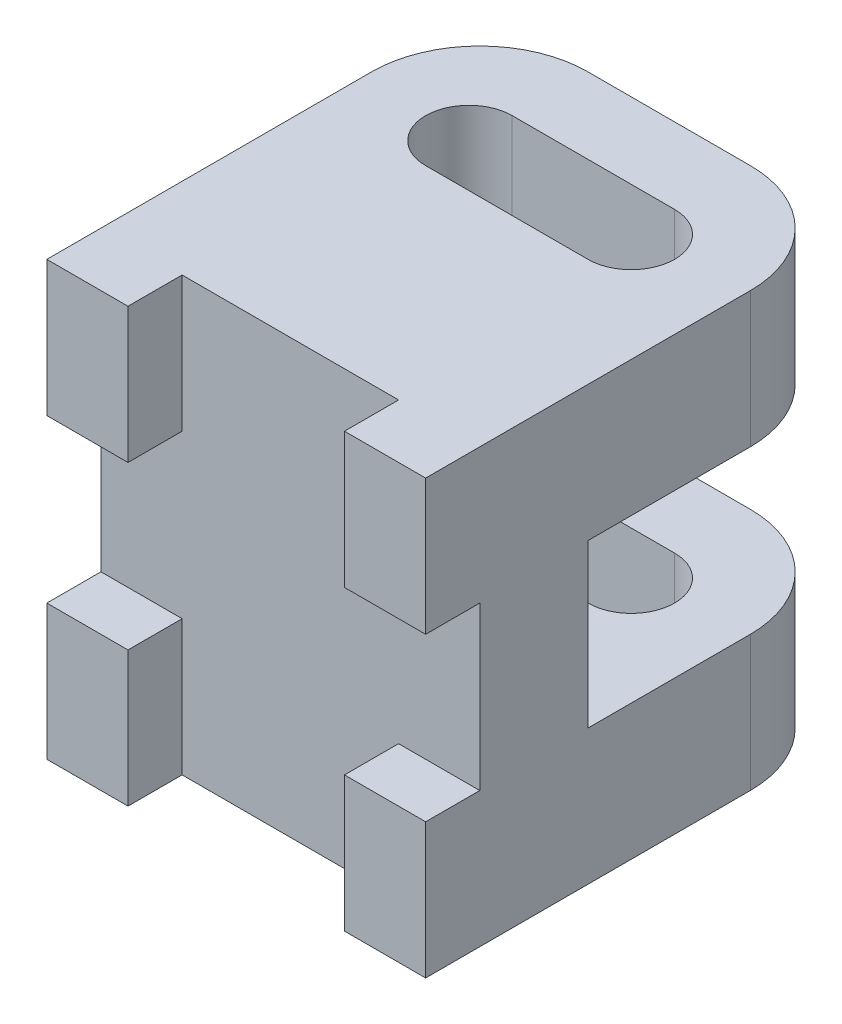
ISO-10303-21;
HEADER;
FILE_DESCRIPTION(('STEP AP214'),'2;1');
FILE_NAME('part.step','',(''),(''),'','','');
FILE_SCHEMA(('AUTOMOTIVE_DESIGN { 1 0 10303 214 1 1 1 1 }'));
ENDSEC;
DATA;
#1=APPLICATION_CONTEXT('core data for automotive mechanical design processes');
#2=APPLICATION_PROTOCOL_DEFINITION('international standard','automotive_design',2000,#1);
#3=PRODUCT_CONTEXT('',#1,'mechanical');
#4=PRODUCT('Part','Part','',(#3));
#5=PRODUCT_RELATED_PRODUCT_CATEGORY('part','',(#4));
#6=PRODUCT_DEFINITION_FORMATION('','',#4);
#7=PRODUCT_DEFINITION_CONTEXT('part definition',#1,'design');
#8=PRODUCT_DEFINITION('design','',#6,#7);
#9=PRODUCT_DEFINITION_SHAPE('','',#8);
#10=(LENGTH_UNIT() NAMED_UNIT(*) SI_UNIT(.MILLI.,.METRE.));
#11=(NAMED_UNIT(*) PLANE_ANGLE_UNIT() SI_UNIT($,.RADIAN.));
#12=(NAMED_UNIT(*) SI_UNIT($,.STERADIAN.) SOLID_ANGLE_UNIT());
#13=UNCERTAINTY_MEASURE_WITH_UNIT(LENGTH_MEASURE(1.E-05),#10,'distance_accuracy_value','');
#14=(GEOMETRIC_REPRESENTATION_CONTEXT(3) GLOBAL_UNCERTAINTY_ASSIGNED_CONTEXT((#13)) GLOBAL_UNIT_ASSIGNED_CONTEXT((#10,
#11,#12)) REPRESENTATION_CONTEXT('',''));
#15=CARTESIAN_POINT('',(0.,0.,0.));
#16=DIRECTION('',(0.,0.,1.));
#17=DIRECTION('',(1.,0.,0.));
#18=AXIS2_PLACEMENT_3D('',#15,#16,#17);
#19=CARTESIAN_POINT('',(0.,80.,20.));
#20=DIRECTION('',(1.,0.,0.));
#21=DIRECTION('',(0.,0.,-1.));
#22=AXIS2_PLACEMENT_3D('',#19,#20,#21);
#23=PLANE('',#22);
#24=DIRECTION('',(0.,-1.,0.));
#25=VECTOR('',#24,1.);
#26=CARTESIAN_POINT('',(0.,100.,-30.));
#27=LINE('',#26,#25);
#28=CARTESIAN_POINT('',(0.,25.,-30.));
#29=VERTEX_POINT('',#28);
#30=CARTESIAN_POINT('',(0.,0.,-30.));
#31=VERTEX_POINT('',#30);
#32=EDGE_CURVE('E506',#29,#31,#27,.T.);
#33=ORIENTED_EDGE('',*,*,#32,.T.);
#34=DIRECTION('',(0.,0.,-1.));
#35=VECTOR('',#34,1.);
#36=CARTESIAN_POINT('',(0.,0.,20.));
#37=LINE('',#36,#35);
#38=CARTESIAN_POINT('',(0.,0.,30.));
#39=VERTEX_POINT('',#38);
#40=EDGE_CURVE('E267',#39,#31,#37,.T.);
#41=ORIENTED_EDGE('',*,*,#40,.F.);
#42=DIRECTION('',(0.,-1.,0.));
#43=VECTOR('',#42,1.);
#44=CARTESIAN_POINT('',(0.,25.,30.));
#45=LINE('',#44,#43);
#46=CARTESIAN_POINT('',(0.,25.,30.));
#47=VERTEX_POINT('',#46);
#48=EDGE_CURVE('E356',#47,#39,#45,.T.);
#49=ORIENTED_EDGE('',*,*,#48,.F.);
#50=DIRECTION('',(0.,0.,-1.));
#51=VECTOR('',#50,1.);
#52=CARTESIAN_POINT('',(0.,25.,30.));
#53=LINE('',#52,#51);
#54=CARTESIAN_POINT('',(0.,25.,20.));
#55=VERTEX_POINT('',#54);
#56=EDGE_CURVE('E369',#47,#55,#53,.T.);
#57=ORIENTED_EDGE('',*,*,#56,.T.);
#58=DIRECTION('',(0.,-1.,0.));
#59=VECTOR('',#58,1.);
#60=CARTESIAN_POINT('',(0.,80.,20.));
#61=LINE('',#60,#59);
#62=CARTESIAN_POINT('',(0.,55.,20.));
#63=VERTEX_POINT('',#62);
#64=EDGE_CURVE('E405',#63,#55,#61,.T.);
#65=ORIENTED_EDGE('',*,*,#64,.F.);
#66=DIRECTION('',(0.,0.,-1.));
#67=VECTOR('',#66,1.);
#68=CARTESIAN_POINT('',(0.,55.,30.));
#69=LINE('',#68,#67);
#70=CARTESIAN_POINT('',(0.,55.,30.));
#71=VERTEX_POINT('',#70);
#72=EDGE_CURVE('E398',#71,#63,#69,.T.);
#73=ORIENTED_EDGE('',*,*,#72,.F.);
#74=DIRECTION('',(0.,-1.,0.));
#75=VECTOR('',#74,1.);
#76=CARTESIAN_POINT('',(0.,80.,30.));
#77=LINE('',#76,#75);
#78=CARTESIAN_POINT('',(0.,80.,30.));
#79=VERTEX_POINT('',#78);
#80=EDGE_CURVE('E380',#79,#71,#77,.T.);
#81=ORIENTED_EDGE('',*,*,#80,.F.);
#82=DIRECTION('',(0.,0.,-1.));
#83=VECTOR('',#82,1.);
#84=CARTESIAN_POINT('',(0.,80.,20.));
#85=LINE('',#84,#83);
#86=CARTESIAN_POINT('',(0.,80.,-30.));
#87=VERTEX_POINT('',#86);
#88=EDGE_CURVE('E414',#79,#87,#85,.T.);
#89=ORIENTED_EDGE('',*,*,#88,.T.);
#90=CARTESIAN_POINT('',(0.,55.,-30.));
#91=VERTEX_POINT('',#90);
#92=EDGE_CURVE('E499',#87,#91,#27,.T.);
#93=ORIENTED_EDGE('',*,*,#92,.T.);
#94=DIRECTION('',(0.,0.,1.));
#95=VECTOR('',#94,1.);
#96=CARTESIAN_POINT('',(0.,55.,-50.));
#97=LINE('',#96,#95);
#98=CARTESIAN_POINT('',(0.,55.,0.));
#99=VERTEX_POINT('',#98);
#100=EDGE_CURVE('E288',#91,#99,#97,.T.);
#101=ORIENTED_EDGE('',*,*,#100,.T.);
#102=DIRECTION('',(0.,-1.,0.));
#103=VECTOR('',#102,1.);
#104=CARTESIAN_POINT('',(0.,80.,0.));
#105=LINE('',#104,#103);
#106=CARTESIAN_POINT('',(0.,25.,0.));
#107=VERTEX_POINT('',#106);
#108=EDGE_CURVE('E402',#99,#107,#105,.T.);
#109=ORIENTED_EDGE('',*,*,#108,.T.);
#110=DIRECTION('',(0.,0.,-1.));
#111=VECTOR('',#110,1.);
#112=CARTESIAN_POINT('',(0.,25.,0.));
#113=LINE('',#112,#111);
#114=EDGE_CURVE('E276',#107,#29,#113,.T.);
#115=ORIENTED_EDGE('',*,*,#114,.T.);
#116=EDGE_LOOP('',(#33,#41,#49,#57,#65,#73,#81,#89,#93,#101,#109,#115));
#117=FACE_BOUND('',#116,.T.);
#118=ADVANCED_FACE('F44',(#117),#23,.F.);
#119=CARTESIAN_POINT('',(0.,55.,-50.));
#120=DIRECTION('',(0.,0.,-1.));
#121=DIRECTION('',(-1.,0.,0.));
#122=AXIS2_PLACEMENT_3D('',#119,#120,#121);
#123=PLANE('',#122);
#124=DIRECTION('',(-1.,0.,0.));
#125=VECTOR('',#124,1.);
#126=CARTESIAN_POINT('',(0.,55.,-50.));
#127=LINE('',#126,#125);
#128=CARTESIAN_POINT('',(50.,55.,-50.));
#129=VERTEX_POINT('',#128);
#130=CARTESIAN_POINT('',(20.,55.,-50.));
#131=VERTEX_POINT('',#130);
#132=EDGE_CURVE('E300',#129,#131,#127,.T.);
#133=ORIENTED_EDGE('',*,*,#132,.T.);
#134=DIRECTION('',(0.,-1.,0.));
#135=VECTOR('',#134,1.);
#136=CARTESIAN_POINT('',(20.,100.,-50.));
#137=LINE('',#136,#135);
#138=CARTESIAN_POINT('',(20.,80.,-50.));
#139=VERTEX_POINT('',#138);
#140=EDGE_CURVE('E66',#139,#131,#137,.T.);
#141=ORIENTED_EDGE('',*,*,#140,.F.);
#142=DIRECTION('',(-1.,0.,0.));
#143=VECTOR('',#142,1.);
#144=CARTESIAN_POINT('',(0.,80.,-50.));
#145=LINE('',#144,#143);
#146=CARTESIAN_POINT('',(50.,80.,-50.));
#147=VERTEX_POINT('',#146);
#148=EDGE_CURVE('E293',#147,#139,#145,.T.);
#149=ORIENTED_EDGE('',*,*,#148,.F.);
#150=DIRECTION('',(0.,-1.,0.));
#151=VECTOR('',#150,1.);
#152=CARTESIAN_POINT('',(50.,100.,-50.));
#153=LINE('',#152,#151);
#154=EDGE_CURVE('E269',#147,#129,#153,.T.);
#155=ORIENTED_EDGE('',*,*,#154,.T.);
#156=EDGE_LOOP('',(#133,#141,#149,#155));
#157=FACE_BOUND('',#156,.T.);
#158=ADVANCED_FACE('F561',(#157),#123,.T.);
#159=CARTESIAN_POINT('',(0.,25.,-50.));
#160=DIRECTION('',(0.,0.,-1.));
#161=DIRECTION('',(-1.,0.,0.));
#162=AXIS2_PLACEMENT_3D('',#159,#160,#161);
#163=PLANE('',#162);
#164=DIRECTION('',(1.,0.,0.));
#165=VECTOR('',#164,1.);
#166=CARTESIAN_POINT('',(0.,0.,-50.));
#167=LINE('',#166,#165);
#168=CARTESIAN_POINT('',(20.,0.,-50.));
#169=VERTEX_POINT('',#168);
#170=CARTESIAN_POINT('',(50.,0.,-50.));
#171=VERTEX_POINT('',#170);
#172=EDGE_CURVE('E270',#169,#171,#167,.T.);
#173=ORIENTED_EDGE('',*,*,#172,.F.);
#174=CARTESIAN_POINT('',(20.,25.,-50.));
#175=VERTEX_POINT('',#174);
#176=EDGE_CURVE('E255',#175,#169,#137,.T.);
#177=ORIENTED_EDGE('',*,*,#176,.F.);
#178=DIRECTION('',(1.,0.,0.));
#179=VECTOR('',#178,1.);
#180=CARTESIAN_POINT('',(0.,25.,-50.));
#181=LINE('',#180,#179);
#182=CARTESIAN_POINT('',(50.,25.,-50.));
#183=VERTEX_POINT('',#182);
#184=EDGE_CURVE('E437',#175,#183,#181,.T.);
#185=ORIENTED_EDGE('',*,*,#184,.T.);
#186=EDGE_CURVE('E274',#183,#171,#153,.T.);
#187=ORIENTED_EDGE('',*,*,#186,.T.);
#188=EDGE_LOOP('',(#173,#177,#185,#187));
#189=FACE_BOUND('',#188,.T.);
#190=ADVANCED_FACE('F271',(#189),#163,.T.);
#191=CARTESIAN_POINT('',(0.,0.,0.));
#192=DIRECTION('',(0.,0.,1.));
#193=DIRECTION('',(1.,0.,0.));
#194=AXIS2_PLACEMENT_3D('',#191,#192,#193);
#195=PLANE('',#194);
#196=DIRECTION('',(-1.,0.,0.));
#197=VECTOR('',#196,1.);
#198=CARTESIAN_POINT('',(70.,25.,0.));
#199=LINE('',#198,#197);
#200=CARTESIAN_POINT('',(70.,25.,0.));
#201=VERTEX_POINT('',#200);
#202=EDGE_CURVE('E273',#201,#107,#199,.T.);
#203=ORIENTED_EDGE('',*,*,#202,.T.);
#204=ORIENTED_EDGE('',*,*,#108,.F.);
#205=DIRECTION('',(1.,0.,0.));
#206=VECTOR('',#205,1.);
#207=CARTESIAN_POINT('',(0.,55.,0.));
#208=LINE('',#207,#206);
#209=CARTESIAN_POINT('',(70.,55.,0.));
#210=VERTEX_POINT('',#209);
#211=EDGE_CURVE('E289',#99,#210,#208,.T.);
#212=ORIENTED_EDGE('',*,*,#211,.T.);
#213=DIRECTION('',(0.,1.,0.));
#214=VECTOR('',#213,1.);
#215=CARTESIAN_POINT('',(70.,0.,0.));
#216=LINE('',#215,#214);
#217=EDGE_CURVE('E403',#201,#210,#216,.T.);
#218=ORIENTED_EDGE('',*,*,#217,.F.);
#219=EDGE_LOOP('',(#203,#204,#212,#218));
#220=FACE_BOUND('',#219,.T.);
#221=ADVANCED_FACE('F516',(#220),#195,.F.);
#222=CARTESIAN_POINT('',(0.,0.,20.));
#223=DIRECTION('',(0.,0.,1.));
#224=DIRECTION('',(1.,0.,0.));
#225=AXIS2_PLACEMENT_3D('',#222,#223,#224);
#226=PLANE('',#225);
#227=DIRECTION('',(0.,-1.,0.));
#228=VECTOR('',#227,1.);
#229=CARTESIAN_POINT('',(55.,0.,20.));
#230=LINE('',#229,#228);
#231=CARTESIAN_POINT('',(55.,25.,20.));
#232=VERTEX_POINT('',#231);
#233=CARTESIAN_POINT('',(55.,0.,20.));
#234=VERTEX_POINT('',#233);
#235=EDGE_CURVE('E310',#232,#234,#230,.T.);
#236=ORIENTED_EDGE('',*,*,#235,.F.);
#237=DIRECTION('',(-1.,0.,0.));
#238=VECTOR('',#237,1.);
#239=CARTESIAN_POINT('',(55.,25.,20.));
#240=LINE('',#239,#238);
#241=CARTESIAN_POINT('',(70.,25.,20.));
#242=VERTEX_POINT('',#241);
#243=EDGE_CURVE('E297',#242,#232,#240,.T.);
#244=ORIENTED_EDGE('',*,*,#243,.F.);
#245=DIRECTION('',(0.,1.,0.));
#246=VECTOR('',#245,1.);
#247=CARTESIAN_POINT('',(70.,0.,20.));
#248=LINE('',#247,#246);
#249=CARTESIAN_POINT('',(70.,55.,20.));
#250=VERTEX_POINT('',#249);
#251=EDGE_CURVE('E410',#242,#250,#248,.T.);
#252=ORIENTED_EDGE('',*,*,#251,.T.);
#253=DIRECTION('',(1.,0.,0.));
#254=VECTOR('',#253,1.);
#255=CARTESIAN_POINT('',(55.,55.,20.));
#256=LINE('',#255,#254);
#257=CARTESIAN_POINT('',(55.,55.,20.));
#258=VERTEX_POINT('',#257);
#259=EDGE_CURVE('E331',#258,#250,#256,.T.);
#260=ORIENTED_EDGE('',*,*,#259,.F.);
#261=DIRECTION('',(0.,-1.,0.));
#262=VECTOR('',#261,1.);
#263=CARTESIAN_POINT('',(55.,80.,20.));
#264=LINE('',#263,#262);
#265=CARTESIAN_POINT('',(55.,80.,20.));
#266=VERTEX_POINT('',#265);
#267=EDGE_CURVE('E329',#266,#258,#264,.T.);
#268=ORIENTED_EDGE('',*,*,#267,.F.);
#269=DIRECTION('',(-1.,0.,0.));
#270=VECTOR('',#269,1.);
#271=CARTESIAN_POINT('',(70.,80.,20.));
#272=LINE('',#271,#270);
#273=CARTESIAN_POINT('',(15.,80.,20.));
#274=VERTEX_POINT('',#273);
#275=EDGE_CURVE('E406',#266,#274,#272,.T.);
#276=ORIENTED_EDGE('',*,*,#275,.T.);
#277=DIRECTION('',(0.,1.,0.));
#278=VECTOR('',#277,1.);
#279=CARTESIAN_POINT('',(15.,80.,20.));
#280=LINE('',#279,#278);
#281=CARTESIAN_POINT('',(15.,55.,20.));
#282=VERTEX_POINT('',#281);
#283=EDGE_CURVE('E382',#282,#274,#280,.T.);
#284=ORIENTED_EDGE('',*,*,#283,.F.);
#285=DIRECTION('',(1.,0.,0.));
#286=VECTOR('',#285,1.);
#287=CARTESIAN_POINT('',(15.,55.,20.));
#288=LINE('',#287,#286);
#289=EDGE_CURVE('E376',#63,#282,#288,.T.);
#290=ORIENTED_EDGE('',*,*,#289,.F.);
#291=ORIENTED_EDGE('',*,*,#64,.T.);
#292=DIRECTION('',(-1.,0.,0.));
#293=VECTOR('',#292,1.);
#294=CARTESIAN_POINT('',(0.,25.,20.));
#295=LINE('',#294,#293);
#296=CARTESIAN_POINT('',(15.,25.,20.));
#297=VERTEX_POINT('',#296);
#298=EDGE_CURVE('E358',#297,#55,#295,.T.);
#299=ORIENTED_EDGE('',*,*,#298,.F.);
#300=DIRECTION('',(0.,1.,0.));
#301=VECTOR('',#300,1.);
#302=CARTESIAN_POINT('',(15.,25.,20.));
#303=LINE('',#302,#301);
#304=CARTESIAN_POINT('',(15.,0.,20.));
#305=VERTEX_POINT('',#304);
#306=EDGE_CURVE('E351',#305,#297,#303,.T.);
#307=ORIENTED_EDGE('',*,*,#306,.F.);
#308=DIRECTION('',(1.,0.,0.));
#309=VECTOR('',#308,1.);
#310=CARTESIAN_POINT('',(0.,0.,20.));
#311=LINE('',#310,#309);
#312=EDGE_CURVE('E404',#305,#234,#311,.T.);
#313=ORIENTED_EDGE('',*,*,#312,.T.);
#314=EDGE_LOOP('',(#236,#244,#252,#260,#268,#276,#284,#290,#291,#299,#307,#313));
#315=FACE_BOUND('',#314,.T.);
#316=ADVANCED_FACE('F539',(#315),#226,.T.);
#317=CARTESIAN_POINT('',(0.,0.,20.));
#318=DIRECTION('',(0.,1.,0.));
#319=DIRECTION('',(0.,0.,1.));
#320=AXIS2_PLACEMENT_3D('',#317,#318,#319);
#321=PLANE('',#320);
#322=DIRECTION('',(1.,0.,0.));
#323=VECTOR('',#322,1.);
#324=CARTESIAN_POINT('',(20.,0.,-36.));
#325=LINE('',#324,#323);
#326=CARTESIAN_POINT('',(20.,0.,-36.));
#327=VERTEX_POINT('',#326);
#328=CARTESIAN_POINT('',(50.,0.,-36.));
#329=VERTEX_POINT('',#328);
#330=EDGE_CURVE('E484',#327,#329,#325,.T.);
#331=ORIENTED_EDGE('',*,*,#330,.F.);
#332=CARTESIAN_POINT('',(20.,0.,-28.));
#333=DIRECTION('',(0.,-1.,0.));
#334=DIRECTION('',(0.,0.,-1.));
#335=AXIS2_PLACEMENT_3D('',#332,#333,#334);
#336=CIRCLE('',#335,8.);
#337=CARTESIAN_POINT('',(20.,0.,-20.));
#338=VERTEX_POINT('',#337);
#339=EDGE_CURVE('E486',#338,#327,#336,.T.);
#340=ORIENTED_EDGE('',*,*,#339,.F.);
#341=DIRECTION('',(-1.,0.,0.));
#342=VECTOR('',#341,1.);
#343=CARTESIAN_POINT('',(20.,0.,-20.));
#344=LINE('',#343,#342);
#345=CARTESIAN_POINT('',(50.,0.,-20.));
#346=VERTEX_POINT('',#345);
#347=EDGE_CURVE('E472',#346,#338,#344,.T.);
#348=ORIENTED_EDGE('',*,*,#347,.F.);
#349=CARTESIAN_POINT('',(50.,0.,-28.));
#350=DIRECTION('',(0.,-1.,0.));
#351=DIRECTION('',(0.,0.,-1.));
#352=AXIS2_PLACEMENT_3D('',#349,#350,#351);
#353=CIRCLE('',#352,8.);
#354=EDGE_CURVE('E485',#329,#346,#353,.T.);
#355=ORIENTED_EDGE('',*,*,#354,.F.);
#356=EDGE_LOOP('',(#331,#340,#348,#355));
#357=FACE_BOUND('',#356,.T.);
#358=ORIENTED_EDGE('',*,*,#40,.T.);
#359=CARTESIAN_POINT('',(20.,0.,-30.));
#360=DIRECTION('',(0.,1.,0.));
#361=DIRECTION('',(0.,0.,-1.));
#362=AXIS2_PLACEMENT_3D('',#359,#360,#361);
#363=CIRCLE('',#362,20.);
#364=EDGE_CURVE('E253',#169,#31,#363,.T.);
#365=ORIENTED_EDGE('',*,*,#364,.F.);
#366=ORIENTED_EDGE('',*,*,#172,.T.);
#367=CARTESIAN_POINT('',(50.,0.,-30.));
#368=DIRECTION('',(0.,1.,0.));
#369=DIRECTION('',(0.,0.,-1.));
#370=AXIS2_PLACEMENT_3D('',#367,#368,#369);
#371=CIRCLE('',#370,20.);
#372=CARTESIAN_POINT('',(70.,0.,-30.));
#373=VERTEX_POINT('',#372);
#374=EDGE_CURVE('E503',#373,#171,#371,.T.);
#375=ORIENTED_EDGE('',*,*,#374,.F.);
#376=DIRECTION('',(0.,0.,-1.));
#377=VECTOR('',#376,1.);
#378=CARTESIAN_POINT('',(70.,0.,20.));
#379=LINE('',#378,#377);
#380=CARTESIAN_POINT('',(70.,0.,30.));
#381=VERTEX_POINT('',#380);
#382=EDGE_CURVE('E419',#381,#373,#379,.T.);
#383=ORIENTED_EDGE('',*,*,#382,.F.);
#384=DIRECTION('',(1.,0.,0.));
#385=VECTOR('',#384,1.);
#386=CARTESIAN_POINT('',(55.,0.,30.));
#387=LINE('',#386,#385);
#388=CARTESIAN_POINT('',(55.,0.,30.));
#389=VERTEX_POINT('',#388);
#390=EDGE_CURVE('E303',#389,#381,#387,.T.);
#391=ORIENTED_EDGE('',*,*,#390,.F.);
#392=DIRECTION('',(0.,0.,-1.));
#393=VECTOR('',#392,1.);
#394=CARTESIAN_POINT('',(55.,0.,30.));
#395=LINE('',#394,#393);
#396=EDGE_CURVE('E312',#389,#234,#395,.T.);
#397=ORIENTED_EDGE('',*,*,#396,.T.);
#398=ORIENTED_EDGE('',*,*,#312,.F.);
#399=DIRECTION('',(0.,0.,-1.));
#400=VECTOR('',#399,1.);
#401=CARTESIAN_POINT('',(15.,0.,30.));
#402=LINE('',#401,#400);
#403=CARTESIAN_POINT('',(15.,0.,30.));
#404=VERTEX_POINT('',#403);
#405=EDGE_CURVE('E361',#404,#305,#402,.T.);
#406=ORIENTED_EDGE('',*,*,#405,.F.);
#407=DIRECTION('',(1.,0.,0.));
#408=VECTOR('',#407,1.);
#409=CARTESIAN_POINT('',(0.,0.,30.));
#410=LINE('',#409,#408);
#411=EDGE_CURVE('E363',#39,#404,#410,.T.);
#412=ORIENTED_EDGE('',*,*,#411,.F.);
#413=EDGE_LOOP('',(#358,#365,#366,#375,#383,#391,#397,#398,#406,#412));
#414=FACE_BOUND('',#413,.T.);
#415=ADVANCED_FACE('F262',(#357,#414),#321,.F.);
#416=CARTESIAN_POINT('',(70.,0.,20.));
#417=DIRECTION('',(-1.,0.,0.));
#418=DIRECTION('',(0.,0.,1.));
#419=AXIS2_PLACEMENT_3D('',#416,#417,#418);
#420=PLANE('',#419);
#421=ORIENTED_EDGE('',*,*,#382,.T.);
#422=DIRECTION('',(0.,-1.,0.));
#423=VECTOR('',#422,1.);
#424=CARTESIAN_POINT('',(70.,100.,-30.));
#425=LINE('',#424,#423);
#426=CARTESIAN_POINT('',(70.,25.,-30.));
#427=VERTEX_POINT('',#426);
#428=EDGE_CURVE('E501',#427,#373,#425,.T.);
#429=ORIENTED_EDGE('',*,*,#428,.F.);
#430=DIRECTION('',(0.,0.,1.));
#431=VECTOR('',#430,1.);
#432=CARTESIAN_POINT('',(70.,25.,-50.));
#433=LINE('',#432,#431);
#434=EDGE_CURVE('E286',#427,#201,#433,.T.);
#435=ORIENTED_EDGE('',*,*,#434,.T.);
#436=ORIENTED_EDGE('',*,*,#217,.T.);
#437=DIRECTION('',(0.,0.,-1.));
#438=VECTOR('',#437,1.);
#439=CARTESIAN_POINT('',(70.,55.,0.));
#440=LINE('',#439,#438);
#441=CARTESIAN_POINT('',(70.,55.,-30.));
#442=VERTEX_POINT('',#441);
#443=EDGE_CURVE('E295',#210,#442,#440,.T.);
#444=ORIENTED_EDGE('',*,*,#443,.T.);
#445=CARTESIAN_POINT('',(70.,80.,-30.));
#446=VERTEX_POINT('',#445);
#447=EDGE_CURVE('E56',#446,#442,#425,.T.);
#448=ORIENTED_EDGE('',*,*,#447,.F.);
#449=DIRECTION('',(0.,0.,-1.));
#450=VECTOR('',#449,1.);
#451=CARTESIAN_POINT('',(70.,80.,20.));
#452=LINE('',#451,#450);
#453=CARTESIAN_POINT('',(70.,80.,30.));
#454=VERTEX_POINT('',#453);
#455=EDGE_CURVE('E420',#454,#446,#452,.T.);
#456=ORIENTED_EDGE('',*,*,#455,.F.);
#457=DIRECTION('',(0.,1.,0.));
#458=VECTOR('',#457,1.);
#459=CARTESIAN_POINT('',(70.,80.,30.));
#460=LINE('',#459,#458);
#461=CARTESIAN_POINT('',(70.,55.,30.));
#462=VERTEX_POINT('',#461);
#463=EDGE_CURVE('E334',#462,#454,#460,.T.);
#464=ORIENTED_EDGE('',*,*,#463,.F.);
#465=DIRECTION('',(0.,0.,-1.));
#466=VECTOR('',#465,1.);
#467=CARTESIAN_POINT('',(70.,55.,30.));
#468=LINE('',#467,#466);
#469=EDGE_CURVE('E336',#462,#250,#468,.T.);
#470=ORIENTED_EDGE('',*,*,#469,.T.);
#471=ORIENTED_EDGE('',*,*,#251,.F.);
#472=DIRECTION('',(0.,0.,-1.));
#473=VECTOR('',#472,1.);
#474=CARTESIAN_POINT('',(70.,25.,30.));
#475=LINE('',#474,#473);
#476=CARTESIAN_POINT('',(70.,25.,30.));
#477=VERTEX_POINT('',#476);
#478=EDGE_CURVE('E324',#477,#242,#475,.T.);
#479=ORIENTED_EDGE('',*,*,#478,.F.);
#480=DIRECTION('',(0.,1.,0.));
#481=VECTOR('',#480,1.);
#482=CARTESIAN_POINT('',(70.,0.,30.));
#483=LINE('',#482,#481);
#484=EDGE_CURVE('E306',#381,#477,#483,.T.);
#485=ORIENTED_EDGE('',*,*,#484,.F.);
#486=EDGE_LOOP('',(#421,#429,#435,#436,#444,#448,#456,#464,#470,#471,#479,#485));
#487=FACE_BOUND('',#486,.T.);
#488=ADVANCED_FACE('F524',(#487),#420,.F.);
#489=CARTESIAN_POINT('',(70.,80.,20.));
#490=DIRECTION('',(0.,-1.,0.));
#491=DIRECTION('',(0.,0.,-1.));
#492=AXIS2_PLACEMENT_3D('',#489,#490,#491);
#493=PLANE('',#492);
#494=DIRECTION('',(-1.,0.,0.));
#495=VECTOR('',#494,1.);
#496=CARTESIAN_POINT('',(70.,80.,-20.));
#497=LINE('',#496,#495);
#498=CARTESIAN_POINT('',(50.,80.,-20.));
#499=VERTEX_POINT('',#498);
#500=CARTESIAN_POINT('',(20.,80.,-20.));
#501=VERTEX_POINT('',#500);
#502=EDGE_CURVE('E449',#499,#501,#497,.T.);
#503=ORIENTED_EDGE('',*,*,#502,.T.);
#504=CARTESIAN_POINT('',(20.,80.,-28.));
#505=DIRECTION('',(0.,-1.,0.));
#506=DIRECTION('',(0.,0.,-1.));
#507=AXIS2_PLACEMENT_3D('',#504,#505,#506);
#508=CIRCLE('',#507,8.);
#509=CARTESIAN_POINT('',(20.,80.,-36.));
#510=VERTEX_POINT('',#509);
#511=EDGE_CURVE('E277',#501,#510,#508,.T.);
#512=ORIENTED_EDGE('',*,*,#511,.T.);
#513=DIRECTION('',(1.,0.,0.));
#514=VECTOR('',#513,1.);
#515=CARTESIAN_POINT('',(70.,80.,-36.));
#516=LINE('',#515,#514);
#517=CARTESIAN_POINT('',(50.,80.,-36.));
#518=VERTEX_POINT('',#517);
#519=EDGE_CURVE('E457',#510,#518,#516,.T.);
#520=ORIENTED_EDGE('',*,*,#519,.T.);
#521=CARTESIAN_POINT('',(50.,80.,-28.));
#522=DIRECTION('',(0.,-1.,0.));
#523=DIRECTION('',(0.,0.,-1.));
#524=AXIS2_PLACEMENT_3D('',#521,#522,#523);
#525=CIRCLE('',#524,8.);
#526=EDGE_CURVE('E451',#518,#499,#525,.T.);
#527=ORIENTED_EDGE('',*,*,#526,.T.);
#528=EDGE_LOOP('',(#503,#512,#520,#527));
#529=FACE_BOUND('',#528,.T.);
#530=ORIENTED_EDGE('',*,*,#148,.T.);
#531=CARTESIAN_POINT('',(20.,80.,-30.));
#532=DIRECTION('',(0.,-1.,0.));
#533=DIRECTION('',(0.,0.,-1.));
#534=AXIS2_PLACEMENT_3D('',#531,#532,#533);
#535=CIRCLE('',#534,20.);
#536=EDGE_CURVE('E489',#139,#87,#535,.F.);
#537=ORIENTED_EDGE('',*,*,#536,.T.);
#538=ORIENTED_EDGE('',*,*,#88,.F.);
#539=DIRECTION('',(-1.,0.,0.));
#540=VECTOR('',#539,1.);
#541=CARTESIAN_POINT('',(0.,80.,30.));
#542=LINE('',#541,#540);
#543=CARTESIAN_POINT('',(15.,80.,30.));
#544=VERTEX_POINT('',#543);
#545=EDGE_CURVE('E383',#544,#79,#542,.T.);
#546=ORIENTED_EDGE('',*,*,#545,.F.);
#547=DIRECTION('',(0.,0.,-1.));
#548=VECTOR('',#547,1.);
#549=CARTESIAN_POINT('',(15.,80.,30.));
#550=LINE('',#549,#548);
#551=EDGE_CURVE('E389',#544,#274,#550,.T.);
#552=ORIENTED_EDGE('',*,*,#551,.T.);
#553=ORIENTED_EDGE('',*,*,#275,.F.);
#554=DIRECTION('',(0.,0.,-1.));
#555=VECTOR('',#554,1.);
#556=CARTESIAN_POINT('',(55.,80.,30.));
#557=LINE('',#556,#555);
#558=CARTESIAN_POINT('',(55.,80.,30.));
#559=VERTEX_POINT('',#558);
#560=EDGE_CURVE('E350',#559,#266,#557,.T.);
#561=ORIENTED_EDGE('',*,*,#560,.F.);
#562=DIRECTION('',(-1.,0.,0.));
#563=VECTOR('',#562,1.);
#564=CARTESIAN_POINT('',(55.,80.,30.));
#565=LINE('',#564,#563);
#566=EDGE_CURVE('E326',#454,#559,#565,.T.);
#567=ORIENTED_EDGE('',*,*,#566,.F.);
#568=ORIENTED_EDGE('',*,*,#455,.T.);
#569=CARTESIAN_POINT('',(50.,80.,-30.));
#570=DIRECTION('',(0.,-1.,0.));
#571=DIRECTION('',(0.,0.,-1.));
#572=AXIS2_PLACEMENT_3D('',#569,#570,#571);
#573=CIRCLE('',#572,20.);
#574=EDGE_CURVE('E492',#446,#147,#573,.F.);
#575=ORIENTED_EDGE('',*,*,#574,.T.);
#576=EDGE_LOOP('',(#530,#537,#538,#546,#552,#553,#561,#567,#568,#575));
#577=FACE_BOUND('',#576,.T.);
#578=ADVANCED_FACE('F604',(#529,#577),#493,.F.);
#579=CARTESIAN_POINT('',(15.,55.,30.));
#580=DIRECTION('',(0.,1.,0.));
#581=DIRECTION('',(0.,0.,1.));
#582=AXIS2_PLACEMENT_3D('',#579,#580,#581);
#583=PLANE('',#582);
#584=ORIENTED_EDGE('',*,*,#289,.T.);
#585=DIRECTION('',(0.,0.,-1.));
#586=VECTOR('',#585,1.);
#587=CARTESIAN_POINT('',(15.,55.,30.));
#588=LINE('',#587,#586);
#589=CARTESIAN_POINT('',(15.,55.,30.));
#590=VERTEX_POINT('',#589);
#591=EDGE_CURVE('E392',#590,#282,#588,.T.);
#592=ORIENTED_EDGE('',*,*,#591,.F.);
#593=DIRECTION('',(1.,0.,0.));
#594=VECTOR('',#593,1.);
#595=CARTESIAN_POINT('',(15.,55.,30.));
#596=LINE('',#595,#594);
#597=EDGE_CURVE('E379',#71,#590,#596,.T.);
#598=ORIENTED_EDGE('',*,*,#597,.F.);
#599=ORIENTED_EDGE('',*,*,#72,.T.);
#600=EDGE_LOOP('',(#584,#592,#598,#599));
#601=FACE_BOUND('',#600,.T.);
#602=ADVANCED_FACE('F611',(#601),#583,.F.);
#603=CARTESIAN_POINT('',(15.,80.,30.));
#604=DIRECTION('',(-1.,0.,0.));
#605=DIRECTION('',(0.,0.,1.));
#606=AXIS2_PLACEMENT_3D('',#603,#604,#605);
#607=PLANE('',#606);
#608=ORIENTED_EDGE('',*,*,#283,.T.);
#609=ORIENTED_EDGE('',*,*,#551,.F.);
#610=DIRECTION('',(0.,1.,0.));
#611=VECTOR('',#610,1.);
#612=CARTESIAN_POINT('',(15.,80.,30.));
#613=LINE('',#612,#611);
#614=EDGE_CURVE('E384',#590,#544,#613,.T.);
#615=ORIENTED_EDGE('',*,*,#614,.F.);
#616=ORIENTED_EDGE('',*,*,#591,.T.);
#617=EDGE_LOOP('',(#608,#609,#615,#616));
#618=FACE_BOUND('',#617,.T.);
#619=ADVANCED_FACE('F606',(#618),#607,.F.);
#620=CARTESIAN_POINT('',(0.,0.,30.));
#621=DIRECTION('',(0.,0.,-1.));
#622=DIRECTION('',(-1.,0.,0.));
#623=AXIS2_PLACEMENT_3D('',#620,#621,#622);
#624=PLANE('',#623);
#625=ORIENTED_EDGE('',*,*,#80,.T.);
#626=ORIENTED_EDGE('',*,*,#597,.T.);
#627=ORIENTED_EDGE('',*,*,#614,.T.);
#628=ORIENTED_EDGE('',*,*,#545,.T.);
#629=EDGE_LOOP('',(#625,#626,#627,#628));
#630=FACE_BOUND('',#629,.T.);
#631=ADVANCED_FACE('F556',(#630),#624,.F.);
#632=CARTESIAN_POINT('',(15.,25.,30.));
#633=DIRECTION('',(-1.,0.,0.));
#634=DIRECTION('',(0.,0.,1.));
#635=AXIS2_PLACEMENT_3D('',#632,#633,#634);
#636=PLANE('',#635);
#637=ORIENTED_EDGE('',*,*,#306,.T.);
#638=DIRECTION('',(0.,0.,-1.));
#639=VECTOR('',#638,1.);
#640=CARTESIAN_POINT('',(15.,25.,30.));
#641=LINE('',#640,#639);
#642=CARTESIAN_POINT('',(15.,25.,30.));
#643=VERTEX_POINT('',#642);
#644=EDGE_CURVE('E373',#643,#297,#641,.T.);
#645=ORIENTED_EDGE('',*,*,#644,.F.);
#646=DIRECTION('',(0.,1.,0.));
#647=VECTOR('',#646,1.);
#648=CARTESIAN_POINT('',(15.,25.,30.));
#649=LINE('',#648,#647);
#650=EDGE_CURVE('E355',#404,#643,#649,.T.);
#651=ORIENTED_EDGE('',*,*,#650,.F.);
#652=ORIENTED_EDGE('',*,*,#405,.T.);
#653=EDGE_LOOP('',(#637,#645,#651,#652));
#654=FACE_BOUND('',#653,.T.);
#655=ADVANCED_FACE('F544',(#654),#636,.F.);
#656=CARTESIAN_POINT('',(0.,25.,30.));
#657=DIRECTION('',(0.,-1.,0.));
#658=DIRECTION('',(0.,0.,-1.));
#659=AXIS2_PLACEMENT_3D('',#656,#657,#658);
#660=PLANE('',#659);
#661=ORIENTED_EDGE('',*,*,#298,.T.);
#662=ORIENTED_EDGE('',*,*,#56,.F.);
#663=DIRECTION('',(-1.,0.,0.));
#664=VECTOR('',#663,1.);
#665=CARTESIAN_POINT('',(0.,25.,30.));
#666=LINE('',#665,#664);
#667=EDGE_CURVE('E354',#643,#47,#666,.T.);
#668=ORIENTED_EDGE('',*,*,#667,.F.);
#669=ORIENTED_EDGE('',*,*,#644,.T.);
#670=EDGE_LOOP('',(#661,#662,#668,#669));
#671=FACE_BOUND('',#670,.T.);
#672=ADVANCED_FACE('F547',(#671),#660,.F.);
#673=CARTESIAN_POINT('',(0.,0.,30.));
#674=DIRECTION('',(0.,0.,1.));
#675=DIRECTION('',(1.,0.,0.));
#676=AXIS2_PLACEMENT_3D('',#673,#674,#675);
#677=PLANE('',#676);
#678=ORIENTED_EDGE('',*,*,#650,.T.);
#679=ORIENTED_EDGE('',*,*,#667,.T.);
#680=ORIENTED_EDGE('',*,*,#48,.T.);
#681=ORIENTED_EDGE('',*,*,#411,.T.);
#682=EDGE_LOOP('',(#678,#679,#680,#681));
#683=FACE_BOUND('',#682,.T.);
#684=ADVANCED_FACE('F545',(#683),#677,.T.);
#685=CARTESIAN_POINT('',(55.,80.,30.));
#686=DIRECTION('',(1.,0.,0.));
#687=DIRECTION('',(0.,0.,-1.));
#688=AXIS2_PLACEMENT_3D('',#685,#686,#687);
#689=PLANE('',#688);
#690=ORIENTED_EDGE('',*,*,#267,.T.);
#691=DIRECTION('',(0.,0.,-1.));
#692=VECTOR('',#691,1.);
#693=CARTESIAN_POINT('',(55.,55.,30.));
#694=LINE('',#693,#692);
#695=CARTESIAN_POINT('',(55.,55.,30.));
#696=VERTEX_POINT('',#695);
#697=EDGE_CURVE('E343',#696,#258,#694,.T.);
#698=ORIENTED_EDGE('',*,*,#697,.F.);
#699=DIRECTION('',(0.,-1.,0.));
#700=VECTOR('',#699,1.);
#701=CARTESIAN_POINT('',(55.,80.,30.));
#702=LINE('',#701,#700);
#703=EDGE_CURVE('E327',#559,#696,#702,.T.);
#704=ORIENTED_EDGE('',*,*,#703,.F.);
#705=ORIENTED_EDGE('',*,*,#560,.T.);
#706=EDGE_LOOP('',(#690,#698,#704,#705));
#707=FACE_BOUND('',#706,.T.);
#708=ADVANCED_FACE('F558',(#707),#689,.F.);
#709=CARTESIAN_POINT('',(55.,55.,30.));
#710=DIRECTION('',(0.,1.,0.));
#711=DIRECTION('',(0.,0.,1.));
#712=AXIS2_PLACEMENT_3D('',#709,#710,#711);
#713=PLANE('',#712);
#714=ORIENTED_EDGE('',*,*,#259,.T.);
#715=ORIENTED_EDGE('',*,*,#469,.F.);
#716=DIRECTION('',(1.,0.,0.));
#717=VECTOR('',#716,1.);
#718=CARTESIAN_POINT('',(55.,55.,30.));
#719=LINE('',#718,#717);
#720=EDGE_CURVE('E333',#696,#462,#719,.T.);
#721=ORIENTED_EDGE('',*,*,#720,.F.);
#722=ORIENTED_EDGE('',*,*,#697,.T.);
#723=EDGE_LOOP('',(#714,#715,#721,#722));
#724=FACE_BOUND('',#723,.T.);
#725=ADVANCED_FACE('F589',(#724),#713,.F.);
#726=CARTESIAN_POINT('',(0.,0.,30.));
#727=DIRECTION('',(0.,0.,-1.));
#728=DIRECTION('',(-1.,0.,0.));
#729=AXIS2_PLACEMENT_3D('',#726,#727,#728);
#730=PLANE('',#729);
#731=ORIENTED_EDGE('',*,*,#566,.T.);
#732=ORIENTED_EDGE('',*,*,#703,.T.);
#733=ORIENTED_EDGE('',*,*,#720,.T.);
#734=ORIENTED_EDGE('',*,*,#463,.T.);
#735=EDGE_LOOP('',(#731,#732,#733,#734));
#736=FACE_BOUND('',#735,.T.);
#737=ADVANCED_FACE('F585',(#736),#730,.F.);
#738=CARTESIAN_POINT('',(55.,25.,30.));
#739=DIRECTION('',(0.,-1.,0.));
#740=DIRECTION('',(0.,0.,-1.));
#741=AXIS2_PLACEMENT_3D('',#738,#739,#740);
#742=PLANE('',#741);
#743=ORIENTED_EDGE('',*,*,#243,.T.);
#744=DIRECTION('',(0.,0.,-1.));
#745=VECTOR('',#744,1.);
#746=CARTESIAN_POINT('',(55.,25.,30.));
#747=LINE('',#746,#745);
#748=CARTESIAN_POINT('',(55.,25.,30.));
#749=VERTEX_POINT('',#748);
#750=EDGE_CURVE('E318',#749,#232,#747,.T.);
#751=ORIENTED_EDGE('',*,*,#750,.F.);
#752=DIRECTION('',(-1.,0.,0.));
#753=VECTOR('',#752,1.);
#754=CARTESIAN_POINT('',(55.,25.,30.));
#755=LINE('',#754,#753);
#756=EDGE_CURVE('E307',#477,#749,#755,.T.);
#757=ORIENTED_EDGE('',*,*,#756,.F.);
#758=ORIENTED_EDGE('',*,*,#478,.T.);
#759=EDGE_LOOP('',(#743,#751,#757,#758));
#760=FACE_BOUND('',#759,.T.);
#761=ADVANCED_FACE('F576',(#760),#742,.F.);
#762=CARTESIAN_POINT('',(55.,0.,30.));
#763=DIRECTION('',(1.,0.,0.));
#764=DIRECTION('',(0.,0.,-1.));
#765=AXIS2_PLACEMENT_3D('',#762,#763,#764);
#766=PLANE('',#765);
#767=ORIENTED_EDGE('',*,*,#235,.T.);
#768=ORIENTED_EDGE('',*,*,#396,.F.);
#769=DIRECTION('',(0.,-1.,0.));
#770=VECTOR('',#769,1.);
#771=CARTESIAN_POINT('',(55.,0.,30.));
#772=LINE('',#771,#770);
#773=EDGE_CURVE('E311',#749,#389,#772,.T.);
#774=ORIENTED_EDGE('',*,*,#773,.F.);
#775=ORIENTED_EDGE('',*,*,#750,.T.);
#776=EDGE_LOOP('',(#767,#768,#774,#775));
#777=FACE_BOUND('',#776,.T.);
#778=ADVANCED_FACE('F531',(#777),#766,.F.);
#779=CARTESIAN_POINT('',(0.,0.,30.));
#780=DIRECTION('',(0.,0.,1.));
#781=DIRECTION('',(1.,0.,0.));
#782=AXIS2_PLACEMENT_3D('',#779,#780,#781);
#783=PLANE('',#782);
#784=ORIENTED_EDGE('',*,*,#390,.T.);
#785=ORIENTED_EDGE('',*,*,#484,.T.);
#786=ORIENTED_EDGE('',*,*,#756,.T.);
#787=ORIENTED_EDGE('',*,*,#773,.T.);
#788=EDGE_LOOP('',(#784,#785,#786,#787));
#789=FACE_BOUND('',#788,.T.);
#790=ADVANCED_FACE('F528',(#789),#783,.T.);
#791=CARTESIAN_POINT('',(0.,55.,0.));
#792=DIRECTION('',(0.,1.,0.));
#793=DIRECTION('',(0.,0.,1.));
#794=AXIS2_PLACEMENT_3D('',#791,#792,#793);
#795=PLANE('',#794);
#796=DIRECTION('',(-1.,0.,0.));
#797=VECTOR('',#796,1.);
#798=CARTESIAN_POINT('',(0.,55.,-36.));
#799=LINE('',#798,#797);
#800=CARTESIAN_POINT('',(50.,55.,-36.));
#801=VERTEX_POINT('',#800);
#802=CARTESIAN_POINT('',(20.,55.,-36.));
#803=VERTEX_POINT('',#802);
#804=EDGE_CURVE('E463',#801,#803,#799,.T.);
#805=ORIENTED_EDGE('',*,*,#804,.T.);
#806=CARTESIAN_POINT('',(20.,55.,-28.));
#807=DIRECTION('',(0.,1.,0.));
#808=DIRECTION('',(0.,0.,1.));
#809=AXIS2_PLACEMENT_3D('',#806,#807,#808);
#810=CIRCLE('',#809,8.);
#811=CARTESIAN_POINT('',(20.,55.,-20.));
#812=VERTEX_POINT('',#811);
#813=EDGE_CURVE('E281',#803,#812,#810,.T.);
#814=ORIENTED_EDGE('',*,*,#813,.T.);
#815=DIRECTION('',(1.,0.,0.));
#816=VECTOR('',#815,1.);
#817=CARTESIAN_POINT('',(0.,55.,-20.));
#818=LINE('',#817,#816);
#819=CARTESIAN_POINT('',(50.,55.,-20.));
#820=VERTEX_POINT('',#819);
#821=EDGE_CURVE('E452',#812,#820,#818,.T.);
#822=ORIENTED_EDGE('',*,*,#821,.T.);
#823=CARTESIAN_POINT('',(50.,55.,-28.));
#824=DIRECTION('',(0.,1.,0.));
#825=DIRECTION('',(0.,0.,1.));
#826=AXIS2_PLACEMENT_3D('',#823,#824,#825);
#827=CIRCLE('',#826,8.);
#828=EDGE_CURVE('E456',#820,#801,#827,.T.);
#829=ORIENTED_EDGE('',*,*,#828,.T.);
#830=EDGE_LOOP('',(#805,#814,#822,#829));
#831=FACE_BOUND('',#830,.T.);
#832=ORIENTED_EDGE('',*,*,#100,.F.);
#833=CARTESIAN_POINT('',(20.,55.,-30.));
#834=DIRECTION('',(0.,1.,0.));
#835=DIRECTION('',(0.,0.,1.));
#836=AXIS2_PLACEMENT_3D('',#833,#834,#835);
#837=CIRCLE('',#836,20.);
#838=EDGE_CURVE('E491',#91,#131,#837,.F.);
#839=ORIENTED_EDGE('',*,*,#838,.T.);
#840=ORIENTED_EDGE('',*,*,#132,.F.);
#841=CARTESIAN_POINT('',(50.,55.,-30.));
#842=DIRECTION('',(0.,1.,0.));
#843=DIRECTION('',(0.,0.,1.));
#844=AXIS2_PLACEMENT_3D('',#841,#842,#843);
#845=CIRCLE('',#844,20.);
#846=EDGE_CURVE('E498',#129,#442,#845,.F.);
#847=ORIENTED_EDGE('',*,*,#846,.T.);
#848=ORIENTED_EDGE('',*,*,#443,.F.);
#849=ORIENTED_EDGE('',*,*,#211,.F.);
#850=EDGE_LOOP('',(#832,#839,#840,#847,#848,#849));
#851=FACE_BOUND('',#850,.T.);
#852=ADVANCED_FACE('F514',(#831,#851),#795,.F.);
#853=CARTESIAN_POINT('',(0.,25.,0.));
#854=DIRECTION('',(0.,-1.,0.));
#855=DIRECTION('',(0.,0.,-1.));
#856=AXIS2_PLACEMENT_3D('',#853,#854,#855);
#857=PLANE('',#856);
#858=DIRECTION('',(-1.,0.,0.));
#859=VECTOR('',#858,1.);
#860=CARTESIAN_POINT('',(0.,25.,-20.));
#861=LINE('',#860,#859);
#862=CARTESIAN_POINT('',(50.,25.,-20.));
#863=VERTEX_POINT('',#862);
#864=CARTESIAN_POINT('',(20.,25.,-20.));
#865=VERTEX_POINT('',#864);
#866=EDGE_CURVE('E427',#863,#865,#861,.T.);
#867=ORIENTED_EDGE('',*,*,#866,.T.);
#868=CARTESIAN_POINT('',(20.,25.,-28.));
#869=DIRECTION('',(0.,-1.,0.));
#870=DIRECTION('',(0.,0.,-1.));
#871=AXIS2_PLACEMENT_3D('',#868,#869,#870);
#872=CIRCLE('',#871,8.);
#873=CARTESIAN_POINT('',(20.,25.,-36.));
#874=VERTEX_POINT('',#873);
#875=EDGE_CURVE('E433',#865,#874,#872,.T.);
#876=ORIENTED_EDGE('',*,*,#875,.T.);
#877=DIRECTION('',(1.,0.,0.));
#878=VECTOR('',#877,1.);
#879=CARTESIAN_POINT('',(0.,25.,-36.));
#880=LINE('',#879,#878);
#881=CARTESIAN_POINT('',(50.,25.,-36.));
#882=VERTEX_POINT('',#881);
#883=EDGE_CURVE('E425',#874,#882,#880,.T.);
#884=ORIENTED_EDGE('',*,*,#883,.T.);
#885=CARTESIAN_POINT('',(50.,25.,-28.));
#886=DIRECTION('',(0.,-1.,0.));
#887=DIRECTION('',(0.,0.,-1.));
#888=AXIS2_PLACEMENT_3D('',#885,#886,#887);
#889=CIRCLE('',#888,8.);
#890=EDGE_CURVE('E430',#882,#863,#889,.T.);
#891=ORIENTED_EDGE('',*,*,#890,.T.);
#892=EDGE_LOOP('',(#867,#876,#884,#891));
#893=FACE_BOUND('',#892,.T.);
#894=ORIENTED_EDGE('',*,*,#184,.F.);
#895=CARTESIAN_POINT('',(20.,25.,-30.));
#896=DIRECTION('',(0.,-1.,0.));
#897=DIRECTION('',(0.,0.,-1.));
#898=AXIS2_PLACEMENT_3D('',#895,#896,#897);
#899=CIRCLE('',#898,20.);
#900=EDGE_CURVE('E11',#175,#29,#899,.F.);
#901=ORIENTED_EDGE('',*,*,#900,.T.);
#902=ORIENTED_EDGE('',*,*,#114,.F.);
#903=ORIENTED_EDGE('',*,*,#202,.F.);
#904=ORIENTED_EDGE('',*,*,#434,.F.);
#905=CARTESIAN_POINT('',(50.,25.,-30.));
#906=DIRECTION('',(0.,-1.,0.));
#907=DIRECTION('',(0.,0.,-1.));
#908=AXIS2_PLACEMENT_3D('',#905,#906,#907);
#909=CIRCLE('',#908,20.);
#910=EDGE_CURVE('E55',#427,#183,#909,.F.);
#911=ORIENTED_EDGE('',*,*,#910,.T.);
#912=EDGE_LOOP('',(#894,#901,#902,#903,#904,#911));
#913=FACE_BOUND('',#912,.T.);
#914=ADVANCED_FACE('F438',(#893,#913),#857,.F.);
#915=CARTESIAN_POINT('',(20.,100.,-36.));
#916=DIRECTION('',(0.,0.,-1.));
#917=DIRECTION('',(-1.,0.,0.));
#918=AXIS2_PLACEMENT_3D('',#915,#916,#917);
#919=PLANE('',#918);
#920=DIRECTION('',(0.,-1.,0.));
#921=VECTOR('',#920,1.);
#922=CARTESIAN_POINT('',(20.,100.,-36.));
#923=LINE('',#922,#921);
#924=EDGE_CURVE('E470',#874,#327,#923,.T.);
#925=ORIENTED_EDGE('',*,*,#924,.T.);
#926=ORIENTED_EDGE('',*,*,#330,.T.);
#927=DIRECTION('',(0.,-1.,0.));
#928=VECTOR('',#927,1.);
#929=CARTESIAN_POINT('',(50.,100.,-36.));
#930=LINE('',#929,#928);
#931=EDGE_CURVE('E475',#882,#329,#930,.T.);
#932=ORIENTED_EDGE('',*,*,#931,.F.);
#933=ORIENTED_EDGE('',*,*,#883,.F.);
#934=EDGE_LOOP('',(#925,#926,#932,#933));
#935=FACE_BOUND('',#934,.T.);
#936=ADVANCED_FACE('F632',(#935),#919,.F.);
#937=CARTESIAN_POINT('',(50.,100.,-28.));
#938=DIRECTION('',(0.,-1.,0.));
#939=DIRECTION('',(0.,0.,-1.));
#940=AXIS2_PLACEMENT_3D('',#937,#938,#939);
#941=CYLINDRICAL_SURFACE('',#940,8.);
#942=ORIENTED_EDGE('',*,*,#931,.T.);
#943=ORIENTED_EDGE('',*,*,#354,.T.);
#944=DIRECTION('',(0.,-1.,0.));
#945=VECTOR('',#944,1.);
#946=CARTESIAN_POINT('',(50.,100.,-20.));
#947=LINE('',#946,#945);
#948=EDGE_CURVE('E473',#863,#346,#947,.T.);
#949=ORIENTED_EDGE('',*,*,#948,.F.);
#950=ORIENTED_EDGE('',*,*,#890,.F.);
#951=EDGE_LOOP('',(#942,#943,#949,#950));
#952=FACE_BOUND('',#951,.T.);
#953=ADVANCED_FACE('F642',(#952),#941,.F.);
#954=CARTESIAN_POINT('',(20.,100.,-20.));
#955=DIRECTION('',(0.,0.,1.));
#956=DIRECTION('',(1.,0.,0.));
#957=AXIS2_PLACEMENT_3D('',#954,#955,#956);
#958=PLANE('',#957);
#959=ORIENTED_EDGE('',*,*,#948,.T.);
#960=ORIENTED_EDGE('',*,*,#347,.T.);
#961=DIRECTION('',(0.,-1.,0.));
#962=VECTOR('',#961,1.);
#963=CARTESIAN_POINT('',(20.,100.,-20.));
#964=LINE('',#963,#962);
#965=EDGE_CURVE('E480',#865,#338,#964,.T.);
#966=ORIENTED_EDGE('',*,*,#965,.F.);
#967=ORIENTED_EDGE('',*,*,#866,.F.);
#968=EDGE_LOOP('',(#959,#960,#966,#967));
#969=FACE_BOUND('',#968,.T.);
#970=ADVANCED_FACE('F646',(#969),#958,.F.);
#971=CARTESIAN_POINT('',(20.,100.,-28.));
#972=DIRECTION('',(0.,-1.,0.));
#973=DIRECTION('',(0.,0.,-1.));
#974=AXIS2_PLACEMENT_3D('',#971,#972,#973);
#975=CYLINDRICAL_SURFACE('',#974,8.);
#976=ORIENTED_EDGE('',*,*,#965,.T.);
#977=ORIENTED_EDGE('',*,*,#339,.T.);
#978=ORIENTED_EDGE('',*,*,#924,.F.);
#979=ORIENTED_EDGE('',*,*,#875,.F.);
#980=EDGE_LOOP('',(#976,#977,#978,#979));
#981=FACE_BOUND('',#980,.T.);
#982=ADVANCED_FACE('F664',(#981),#975,.F.);
#983=EDGE_CURVE('E467',#501,#812,#964,.T.);
#984=ORIENTED_EDGE('',*,*,#983,.T.);
#985=ORIENTED_EDGE('',*,*,#813,.F.);
#986=EDGE_CURVE('E468',#510,#803,#923,.T.);
#987=ORIENTED_EDGE('',*,*,#986,.F.);
#988=ORIENTED_EDGE('',*,*,#511,.F.);
#989=EDGE_LOOP('',(#984,#985,#987,#988));
#990=FACE_BOUND('',#989,.T.);
#991=ADVANCED_FACE('F668',(#990),#975,.F.);
#992=EDGE_CURVE('E476',#499,#820,#947,.T.);
#993=ORIENTED_EDGE('',*,*,#992,.T.);
#994=ORIENTED_EDGE('',*,*,#821,.F.);
#995=ORIENTED_EDGE('',*,*,#983,.F.);
#996=ORIENTED_EDGE('',*,*,#502,.F.);
#997=EDGE_LOOP('',(#993,#994,#995,#996));
#998=FACE_BOUND('',#997,.T.);
#999=ADVANCED_FACE('F637',(#998),#958,.F.);
#1000=EDGE_CURVE('E471',#518,#801,#930,.T.);
#1001=ORIENTED_EDGE('',*,*,#1000,.T.);
#1002=ORIENTED_EDGE('',*,*,#828,.F.);
#1003=ORIENTED_EDGE('',*,*,#992,.F.);
#1004=ORIENTED_EDGE('',*,*,#526,.F.);
#1005=EDGE_LOOP('',(#1001,#1002,#1003,#1004));
#1006=FACE_BOUND('',#1005,.T.);
#1007=ADVANCED_FACE('F631',(#1006),#941,.F.);
#1008=ORIENTED_EDGE('',*,*,#986,.T.);
#1009=ORIENTED_EDGE('',*,*,#804,.F.);
#1010=ORIENTED_EDGE('',*,*,#1000,.F.);
#1011=ORIENTED_EDGE('',*,*,#519,.F.);
#1012=EDGE_LOOP('',(#1008,#1009,#1010,#1011));
#1013=FACE_BOUND('',#1012,.T.);
#1014=ADVANCED_FACE('F630',(#1013),#919,.F.);
#1015=CARTESIAN_POINT('',(50.,100.,-30.));
#1016=DIRECTION('',(0.,-1.,0.));
#1017=DIRECTION('',(0.,0.,-1.));
#1018=AXIS2_PLACEMENT_3D('',#1015,#1016,#1017);
#1019=CYLINDRICAL_SURFACE('',#1018,20.);
#1020=ORIENTED_EDGE('',*,*,#428,.T.);
#1021=ORIENTED_EDGE('',*,*,#374,.T.);
#1022=ORIENTED_EDGE('',*,*,#186,.F.);
#1023=ORIENTED_EDGE('',*,*,#910,.F.);
#1024=EDGE_LOOP('',(#1020,#1021,#1022,#1023));
#1025=FACE_BOUND('',#1024,.T.);
#1026=ADVANCED_FACE('F525',(#1025),#1019,.T.);
#1027=CARTESIAN_POINT('',(20.,100.,-30.));
#1028=DIRECTION('',(0.,-1.,0.));
#1029=DIRECTION('',(0.,0.,-1.));
#1030=AXIS2_PLACEMENT_3D('',#1027,#1028,#1029);
#1031=CYLINDRICAL_SURFACE('',#1030,20.);
#1032=ORIENTED_EDGE('',*,*,#176,.T.);
#1033=ORIENTED_EDGE('',*,*,#364,.T.);
#1034=ORIENTED_EDGE('',*,*,#32,.F.);
#1035=ORIENTED_EDGE('',*,*,#900,.F.);
#1036=EDGE_LOOP('',(#1032,#1033,#1034,#1035));
#1037=FACE_BOUND('',#1036,.T.);
#1038=ADVANCED_FACE('F251',(#1037),#1031,.T.);
#1039=ORIENTED_EDGE('',*,*,#447,.T.);
#1040=ORIENTED_EDGE('',*,*,#846,.F.);
#1041=ORIENTED_EDGE('',*,*,#154,.F.);
#1042=ORIENTED_EDGE('',*,*,#574,.F.);
#1043=EDGE_LOOP('',(#1039,#1040,#1041,#1042));
#1044=FACE_BOUND('',#1043,.T.);
#1045=ADVANCED_FACE('F618',(#1044),#1019,.T.);
#1046=ORIENTED_EDGE('',*,*,#140,.T.);
#1047=ORIENTED_EDGE('',*,*,#838,.F.);
#1048=ORIENTED_EDGE('',*,*,#92,.F.);
#1049=ORIENTED_EDGE('',*,*,#536,.F.);
#1050=EDGE_LOOP('',(#1046,#1047,#1048,#1049));
#1051=FACE_BOUND('',#1050,.T.);
#1052=ADVANCED_FACE('F612',(#1051),#1031,.T.);
#1053=CLOSED_SHELL('',(#118,#158,#190,#221,#316,#415,#488,#578,#602,#619,#631,#655,#672,#684,
#708,#725,#737,#761,#778,#790,#852,#914,#936,#953,#970,#982,#991,#999,#1007,#1014,#1026,#1038,
#1045,#1052));
#1054=MANIFOLD_SOLID_BREP('B2',#1053);
#1055=ADVANCED_BREP_SHAPE_REPRESENTATION('',(#18,#1054),#14);
#1056=SHAPE_DEFINITION_REPRESENTATION(#9,#1055);
ENDSEC;
END-ISO-10303-21;
